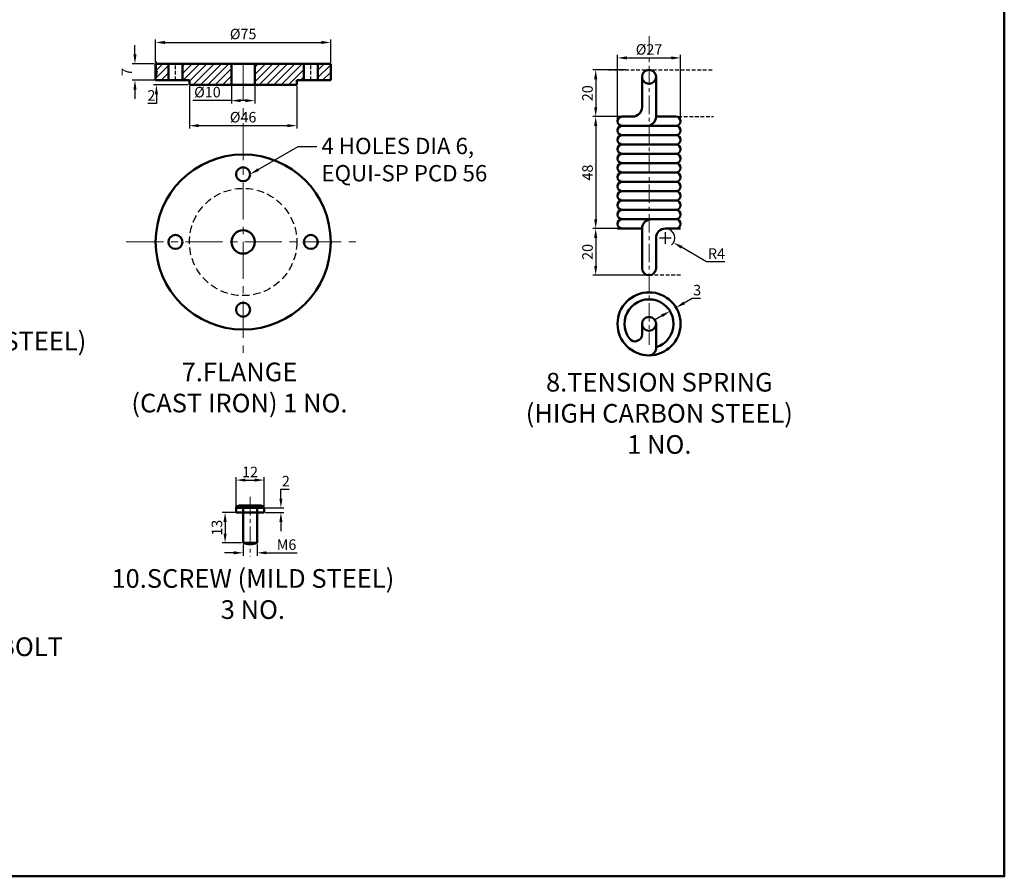
# Model space of a CAD drawing. Units: millimetres. Extents: x -166 to 681, y -4360 to 126.
# Tile 6 of 7: x 259 to 681, y -430 to -63. Entities that reach past the tile are written whole.
import ezdxf
from ezdxf import colors
from ezdxf.entities.mleader import LeaderData, LeaderLine
from ezdxf.math import Vec2, Vec3

# ---------------------------------------------------------------- set-up
doc = ezdxf.new("R2010")
doc.units = ezdxf.units.MM
doc.header["$LTSCALE"] = 0.5
doc.linetypes.add('CENTER', pattern=[50.8, 31.75, -6.35, 6.35, -6.35])
doc.linetypes.add('HIDDEN', pattern=[9.525, 6.35, -3.175])
for name, color, linetype, lineweight in [('M-CNTR', 1, 'CENTER', 18), ('M-DIMS', 2, 'Continuous', 25), ('M-HATC', 8, 'Continuous', 18), ('M-HIDN', 3, 'HIDDEN', 25), ('M-OUTL', 7, 'Continuous', 50), ('M-TEXT', 7, 'Continuous', 25), ('M-TTLB', 7, 'Continuous', 50)]:
    doc.layers.add(name, color=color, linetype=linetype, lineweight=lineweight)
doc.styles.get("Standard").update_dxf_attribs({"font": 'arial.ttf'})
doc.dimstyles.new('ISO-25', dxfattribs={"dimtxt": 4.5, "dimasz": 4, "dimexe": 1.25, "dimexo": 0.625, "dimtad": 1, "dimtoh": 1, "dimdec": 1, "dimtxsty": 'Standard', "dimcen": 2.5, "dimadec": 0, "dimazin": 0, "dimtfac": 1, "dimtdec": 1, "dimtofl": 0, "dimtmove": 0, "dimatfit": 3, "dimfxl": 1, "dimarcsym": 0})

# ---------------------------------------------------------------- blocks, each defined once
blk = doc.blocks.new('*D48')
at = {"layer": 'Defpoints', "color": 0, "ltscale": 0.5, "transparency": 16777216}
for p in [(392.3, -72.72), (317.3, -81.87), (392.3, -81.87)]:
    blk.add_point(p, dxfattribs=at)
at = {"layer": 'M-DIMS', "color": 0, "lineweight": -2, "ltscale": 0.5, "transparency": 16777216}
for p, q in [((317.3, -81.25), (317.3, -71.47)), ((392.3, -81.25), (392.3, -71.47)), ((321.3, -72.72), (388.3, -72.72))]:
    blk.add_line(p, q, dxfattribs=at)
at = {"layer": 'M-DIMS', "color": 0, "ltscale": 0.5, "transparency": 16777216}
for points in [[(321.3, -72.05), (321.3, -73.38), (317.3, -72.72)], [(388.3, -72.05), (388.3, -73.38), (392.3, -72.72)]]:
    blk.add_solid(points, dxfattribs=at)
at = {"layer": 'M-DIMS', "color": 0, "ltscale": 0.5, "transparency": 16777216, "insert": (354.8, -69.67), "char_height": 4.5, "attachment_point": 5}
blk.add_mtext('%%C75', dxfattribs=at)
blk = doc.blocks.new('*D49')
at = {"layer": 'Defpoints', "color": 0, "ltscale": 0.5, "transparency": 16777216}
for p in [(317.3, -81.87), (308.48, -88.87), (317.3, -88.87)]:
    blk.add_point(p, dxfattribs=at)
at = {"layer": 'M-DIMS', "color": 0, "lineweight": -2, "ltscale": 0.5, "transparency": 16777216}
for p, q in [((308.48, -77.87), (308.48, -73.87)), ((316.67, -81.87), (307.23, -81.87)), ((316.67, -88.87), (307.23, -88.87)), ((308.48, -92.87), (308.48, -96.87))]:
    blk.add_line(p, q, dxfattribs=at)
at = {"layer": 'M-DIMS', "color": 0, "ltscale": 0.5, "transparency": 16777216}
for points in [[(307.82, -77.87), (309.15, -77.87), (308.48, -81.87)], [(307.82, -92.87), (309.15, -92.87), (308.48, -88.87)]]:
    blk.add_solid(points, dxfattribs=at)
at = {"layer": 'M-DIMS', "color": 0, "ltscale": 0.5, "transparency": 16777216, "insert": (305.61, -85.37), "char_height": 4.5, "attachment_point": 5, "rotation": 90}
blk.add_mtext('7', dxfattribs=at)
blk = doc.blocks.new('*D50')
at = {"layer": 'Defpoints', "color": 0, "ltscale": 0.5, "transparency": 16777216}
for p in [(317.66, -90.87), (331.8, -88.87), (331.8, -90.87)]:
    blk.add_point(p, dxfattribs=at)
at = {"layer": 'M-DIMS', "color": 0, "lineweight": -2, "ltscale": 0.5, "transparency": 16777216}
for p, q in [((317.66, -84.87), (317.66, -80.87)), ((331.17, -88.87), (316.41, -88.87)), ((331.17, -90.87), (316.41, -90.87)), ((317.66, -94.87), (317.66, -98.87)), ((317.66, -98.87), (314.05, -98.87))]:
    blk.add_line(p, q, dxfattribs=at)
at = {"layer": 'M-DIMS', "color": 0, "ltscale": 0.5, "transparency": 16777216}
for points in [[(316.99, -84.87), (318.33, -84.87), (317.66, -88.87)], [(316.99, -94.87), (318.33, -94.87), (317.66, -90.87)]]:
    blk.add_solid(points, dxfattribs=at)
at = {"layer": 'M-DIMS', "color": 0, "ltscale": 0.5, "transparency": 16777216, "insert": (315.54, -95.99), "char_height": 4.5, "attachment_point": 5}
blk.add_mtext('2', dxfattribs=at)
blk = doc.blocks.new('*D51')
at = {"layer": 'Defpoints', "color": 0, "ltscale": 0.5, "transparency": 16777216}
for p in [(349.8, -90.87), (359.8, -90.87), (359.8, -97.63)]:
    blk.add_point(p, dxfattribs=at)
at = {"layer": 'M-DIMS', "color": 0, "lineweight": -2, "ltscale": 0.5, "transparency": 16777216}
for p, q in [((349.8, -91.5), (349.8, -98.88)), ((359.8, -91.5), (359.8, -98.88)), ((349.8, -97.63), (333.22, -97.63)), ((355.8, -97.63), (353.8, -97.63))]:
    blk.add_line(p, q, dxfattribs=at)
at = {"layer": 'M-DIMS', "color": 0, "ltscale": 0.5, "transparency": 16777216}
for points in [[(353.8, -96.97), (353.8, -98.3), (349.8, -97.63)], [(355.8, -96.97), (355.8, -98.3), (359.8, -97.63)]]:
    blk.add_solid(points, dxfattribs=at)
at = {"layer": 'M-DIMS', "color": 0, "ltscale": 0.5, "transparency": 16777216, "insert": (339.51, -94.58), "char_height": 4.5, "attachment_point": 5}
blk.add_mtext('%%C10', dxfattribs=at)
blk = doc.blocks.new('*D52')
at = {"layer": 'Defpoints', "color": 0, "ltscale": 0.5, "transparency": 16777216}
for p in [(331.8, -90.87), (377.8, -90.87), (377.8, -108.36)]:
    blk.add_point(p, dxfattribs=at)
at = {"layer": 'M-DIMS', "color": 0, "lineweight": -2, "ltscale": 0.5, "transparency": 16777216}
for p, q in [((331.8, -91.5), (331.8, -109.61)), ((377.8, -91.5), (377.8, -109.61)), ((335.8, -108.36), (373.8, -108.36))]:
    blk.add_line(p, q, dxfattribs=at)
at = {"layer": 'M-DIMS', "color": 0, "ltscale": 0.5, "transparency": 16777216}
for points in [[(335.8, -107.7), (335.8, -109.03), (331.8, -108.36)], [(373.8, -107.7), (373.8, -109.03), (377.8, -108.36)]]:
    blk.add_solid(points, dxfattribs=at)
at = {"layer": 'M-DIMS', "color": 0, "ltscale": 0.5, "transparency": 16777216, "insert": (354.8, -105.31), "char_height": 4.5, "attachment_point": 5}
blk.add_mtext('%%C46', dxfattribs=at)
blk = doc.blocks.new('*D55')
at = {"layer": 'Defpoints', "color": 0, "ltscale": 0.5, "transparency": 16777216}
for p in [(354.78, -274.15), (347.08, -287.15), (354.78, -287.15)]:
    blk.add_point(p, dxfattribs=at)
at = {"layer": 'M-DIMS', "color": 0, "lineweight": -2, "ltscale": 0.5, "transparency": 16777216}
for p, q in [((354.16, -274.15), (345.83, -274.15)), ((347.08, -278.15), (347.08, -283.15)), ((354.16, -287.15), (345.83, -287.15))]:
    blk.add_line(p, q, dxfattribs=at)
at = {"layer": 'M-DIMS', "color": 0, "ltscale": 0.5, "transparency": 16777216}
for points in [[(346.41, -278.15), (347.75, -278.15), (347.08, -274.15)], [(346.41, -283.15), (347.75, -283.15), (347.08, -287.15)]]:
    blk.add_solid(points, dxfattribs=at)
at = {"layer": 'M-DIMS', "color": 0, "ltscale": 0.5, "transparency": 16777216, "insert": (344.16, -280.65), "char_height": 4.5, "attachment_point": 5, "rotation": 90}
blk.add_mtext('13', dxfattribs=at)
blk = doc.blocks.new('*D56')
at = {"layer": 'Defpoints', "color": 0, "ltscale": 0.5, "transparency": 16777216}
for p in [(354.78, -287.15), (360.78, -287.15), (360.78, -291.39)]:
    blk.add_point(p, dxfattribs=at)
at = {"layer": 'M-DIMS', "color": 0, "lineweight": -2, "ltscale": 0.5, "transparency": 16777216}
for p, q in [((354.78, -287.77), (354.78, -292.64)), ((360.78, -287.77), (360.78, -292.64)), ((350.78, -291.39), (346.78, -291.39)), ((364.78, -291.39), (378.01, -291.39))]:
    blk.add_line(p, q, dxfattribs=at)
at = {"layer": 'M-DIMS', "color": 0, "ltscale": 0.5, "transparency": 16777216}
for points in [[(350.78, -290.72), (350.78, -292.06), (354.78, -291.39)], [(364.78, -290.72), (364.78, -292.06), (360.78, -291.39)]]:
    blk.add_solid(points, dxfattribs=at)
at = {"layer": 'M-DIMS', "color": 0, "ltscale": 0.5, "transparency": 16777216, "insert": (373.4, -288.47), "char_height": 4.5, "attachment_point": 5}
blk.add_mtext('M6', dxfattribs=at)
blk = doc.blocks.new('*D63')
at = {"layer": 'Defpoints', "color": 0, "ltscale": 0.5, "transparency": 16777216}
for p in [(542.14, -79.33), (515.14, -106.43), (542.14, -106.43)]:
    blk.add_point(p, dxfattribs=at)
at = {"layer": 'M-DIMS', "color": 0, "lineweight": -2, "ltscale": 0.5, "transparency": 16777216}
for p, q in [((515.14, -105.8), (515.14, -78.08)), ((519.14, -79.33), (538.14, -79.33)), ((542.14, -105.8), (542.14, -78.08))]:
    blk.add_line(p, q, dxfattribs=at)
at = {"layer": 'M-DIMS', "color": 0, "ltscale": 0.5, "transparency": 16777216}
for points in [[(519.14, -78.67), (519.14, -80), (515.14, -79.33)], [(538.14, -78.67), (538.14, -80), (542.14, -79.33)]]:
    blk.add_solid(points, dxfattribs=at)
at = {"layer": 'M-DIMS', "color": 0, "ltscale": 0.5, "transparency": 16777216, "insert": (528.64, -76.28), "char_height": 4.5, "attachment_point": 5}
blk.add_mtext('%%C27', dxfattribs=at)
blk = doc.blocks.new('*D64')
at = {"layer": 'Defpoints', "color": 0, "ltscale": 0.5, "transparency": 16777216}
for p in [(519.16, -84.46), (505.8, -104.46), (519.39, -104.46)]:
    blk.add_point(p, dxfattribs=at)
at = {"layer": 'M-DIMS', "color": 0, "lineweight": -2, "ltscale": 0.5, "transparency": 16777216}
for p, q in [((518.53, -84.46), (504.55, -84.46)), ((505.8, -88.46), (505.8, -100.46)), ((518.77, -104.46), (504.55, -104.46))]:
    blk.add_line(p, q, dxfattribs=at)
at = {"layer": 'M-DIMS', "color": 0, "ltscale": 0.5, "transparency": 16777216}
for points in [[(505.13, -88.46), (506.46, -88.46), (505.8, -84.46)], [(505.13, -100.46), (506.46, -100.46), (505.8, -104.46)]]:
    blk.add_solid(points, dxfattribs=at)
at = {"layer": 'M-DIMS', "color": 0, "ltscale": 0.5, "transparency": 16777216, "insert": (502.87, -94.46), "char_height": 4.5, "attachment_point": 5, "rotation": 90}
blk.add_mtext('20', dxfattribs=at)
blk = doc.blocks.new('*D65')
at = {"layer": 'Defpoints', "color": 0, "ltscale": 0.5, "transparency": 16777216}
for p in [(511.66, -104.46), (505.8, -152.46), (517.14, -152.46)]:
    blk.add_point(p, dxfattribs=at)
at = {"layer": 'M-DIMS', "color": 0, "lineweight": -2, "ltscale": 0.5, "transparency": 16777216}
for p, q in [((511.03, -104.46), (504.55, -104.46)), ((505.8, -108.46), (505.8, -148.46)), ((516.52, -152.46), (504.55, -152.46))]:
    blk.add_line(p, q, dxfattribs=at)
at = {"layer": 'M-DIMS', "color": 0, "ltscale": 0.5, "transparency": 16777216}
for points in [[(505.13, -108.46), (506.46, -108.46), (505.8, -104.46)], [(505.13, -148.46), (506.46, -148.46), (505.8, -152.46)]]:
    blk.add_solid(points, dxfattribs=at)
at = {"layer": 'M-DIMS', "color": 0, "ltscale": 0.5, "transparency": 16777216, "insert": (502.87, -128.46), "char_height": 4.5, "attachment_point": 5, "rotation": 90}
blk.add_mtext('48', dxfattribs=at)
blk = doc.blocks.new('*D66')
at = {"layer": 'Defpoints', "color": 0, "ltscale": 0.5, "transparency": 16777216}
for p in [(520.39, -152.46), (505.8, -172.46), (528.64, -172.46)]:
    blk.add_point(p, dxfattribs=at)
at = {"layer": 'M-DIMS', "color": 0, "lineweight": -2, "ltscale": 0.5, "transparency": 16777216}
for p, q in [((519.77, -152.46), (504.55, -152.46)), ((505.8, -156.46), (505.8, -168.46)), ((528.02, -172.46), (504.55, -172.46))]:
    blk.add_line(p, q, dxfattribs=at)
at = {"layer": 'M-DIMS', "color": 0, "ltscale": 0.5, "transparency": 16777216}
for points in [[(505.13, -156.46), (506.46, -156.46), (505.8, -152.46)], [(505.13, -168.46), (506.46, -168.46), (505.8, -172.46)]]:
    blk.add_solid(points, dxfattribs=at)
at = {"layer": 'M-DIMS', "color": 0, "ltscale": 0.5, "transparency": 16777216, "insert": (502.87, -162.46), "char_height": 4.5, "attachment_point": 5, "rotation": 90}
blk.add_mtext('20', dxfattribs=at)
blk = doc.blocks.new('*D67')
at = {"layer": 'Defpoints', "color": 0, "ltscale": 0.5, "transparency": 16777216}
for p in [(535.64, -156.46), (539.1, -158.46)]:
    blk.add_point(p, dxfattribs=at)
at = {"layer": 'M-DIMS', "color": 0, "lineweight": -2, "ltscale": 0.5, "transparency": 16777216}
for p, q in [((535.64, -158.96), (535.64, -153.96)), ((533.14, -156.46), (538.14, -156.46)), ((553.28, -166.64), (542.57, -160.46)), ((561.14, -166.64), (553.28, -166.64))]:
    blk.add_line(p, q, dxfattribs=at)
blk.add_arc((535.64, -156.46), 4, 312.0951, 81.0475, dxfattribs=at)
at = {"layer": 'M-DIMS', "color": 0, "ltscale": 0.5, "transparency": 16777216}
blk.add_solid([(542.9, -159.88), (542.24, -161.04), (539.1, -158.46)], dxfattribs=at)
at = {"layer": 'M-DIMS', "color": 0, "ltscale": 0.5, "transparency": 16777216, "insert": (557.52, -163.77), "char_height": 4.5, "attachment_point": 5}
blk.add_mtext('R4', dxfattribs=at)
blk = doc.blocks.new('*D68')
at = {"layer": 'Defpoints', "color": 0, "ltscale": 0.5, "transparency": 16777216}
for p in [(537.62, -187.84), (540.22, -186.34), (540.22, -186.34)]:
    blk.add_point(p, dxfattribs=at)
at = {"layer": 'M-DIMS', "color": 0, "lineweight": -2, "ltscale": 0.5, "transparency": 16777216}
for p, q in [((543.68, -184.34), (547.14, -182.34)), ((547.14, -182.34), (550.72, -182.34)), ((537.93, -188.38), (538.24, -188.92)), ((540.53, -186.88), (540.84, -187.42)), ((534.15, -189.84), (530.69, -191.84))]:
    blk.add_line(p, q, dxfattribs=at)
at = {"layer": 'M-DIMS', "color": 0, "ltscale": 0.5, "transparency": 16777216}
for points in [[(543.35, -183.76), (544.01, -184.91), (540.22, -186.34)], [(533.82, -189.26), (534.49, -190.41), (537.62, -187.84)]]:
    blk.add_solid(points, dxfattribs=at)
at = {"layer": 'M-DIMS', "color": 0, "ltscale": 0.5, "transparency": 16777216, "insert": (549.24, -179.41), "char_height": 4.5, "attachment_point": 5}
blk.add_mtext('3', dxfattribs=at)
blk = doc.blocks.new('*D87')
at = {"layer": 'Defpoints', "color": 0, "ltscale": 0.5, "transparency": 16777216}
for p in [(363.78, -260.23), (351.78, -274.15), (363.78, -274.15)]:
    blk.add_point(p, dxfattribs=at)
at = {"layer": 'M-DIMS', "color": 0, "lineweight": -2, "ltscale": 0.5, "transparency": 16777216}
for p, q in [((351.78, -273.52), (351.78, -258.98)), ((355.78, -260.23), (359.78, -260.23)), ((363.78, -273.52), (363.78, -258.98))]:
    blk.add_line(p, q, dxfattribs=at)
at = {"layer": 'M-DIMS', "color": 0, "ltscale": 0.5, "transparency": 16777216}
for points in [[(355.78, -259.56), (355.78, -260.89), (351.78, -260.23)], [(359.78, -259.56), (359.78, -260.89), (363.78, -260.23)]]:
    blk.add_solid(points, dxfattribs=at)
at = {"layer": 'M-DIMS', "color": 0, "ltscale": 0.5, "transparency": 16777216, "insert": (357.78, -257.34), "char_height": 4.5, "attachment_point": 5}
blk.add_mtext('12', dxfattribs=at)
blk = doc.blocks.new('*D88')
at = {"layer": 'Defpoints', "color": 0, "ltscale": 0.5, "transparency": 16777216}
for p in [(363.78, -272.15), (370.98, -272.15), (363.78, -274.15)]:
    blk.add_point(p, dxfattribs=at)
at = {"layer": 'M-DIMS', "color": 0, "lineweight": -2, "ltscale": 0.5, "transparency": 16777216}
for p, q in [((370.98, -268.15), (370.98, -264.15)), ((370.98, -264.15), (374.59, -264.15)), ((364.41, -272.15), (372.23, -272.15)), ((364.41, -274.15), (372.23, -274.15)), ((370.98, -278.15), (370.98, -282.15))]:
    blk.add_line(p, q, dxfattribs=at)
at = {"layer": 'M-DIMS', "color": 0, "ltscale": 0.5, "transparency": 16777216}
for points in [[(370.32, -268.15), (371.65, -268.15), (370.98, -272.15)], [(370.32, -278.15), (371.65, -278.15), (370.98, -274.15)]]:
    blk.add_solid(points, dxfattribs=at)
at = {"layer": 'M-DIMS', "color": 0, "ltscale": 0.5, "transparency": 16777216, "insert": (373.1, -261.26), "char_height": 4.5, "attachment_point": 5}
blk.add_mtext('2', dxfattribs=at)

msp = doc.modelspace()

# ---------------------------------------------------------------- hatches: boundary and pattern name
at = {"layer": 'M-HATC', "ltscale": 0.5}
h = msp.add_hatch(dxfattribs=at)
h.set_pattern_fill('ANSI31', color=256, scale=0.7)
h.set_pattern_definition([(45, (-558522.521, -290240.8901), (-1.571544821, 1.571544821), [])])
h.paths.add_polyline_path([(322.7995, -88.8706), (322.7995, -81.8706), (317.2995, -81.8706), (317.2995, -88.8706)])
h.paths.add_polyline_path([(349.7995, -90.8706), (349.7995, -81.8706), (328.7995, -81.8706), (328.7995, -88.8706), (331.7995, -88.8706), (331.7995, -90.8706)])
h.paths.add_polyline_path([(377.7995, -90.8706), (377.7995, -88.8706), (380.7995, -88.8706), (380.7995, -81.8706), (359.7995, -81.8706), (359.7995, -90.8706)])
h.paths.add_polyline_path([(392.2995, -81.8706), (386.7995, -81.8706), (386.7995, -88.8706), (392.2995, -88.8706)])

# ---------------------------------------------------------------- linework, layer by layer
at = {"layer": 'M-CNTR', "ltscale": 0.5}
for p, q in [((528.6407, -70.0538), (528.6407, -202.215)), ((357.782, -267.4267), (357.782, -292.9023))]:
    msp.add_line(p, q, dxfattribs=at)
at = {"layer": 'M-CNTR'}
for p, q in [((354.7995, -81.8706), (354.7995, -207.9941)), ((304.7638, -158.2074), (403.0861, -158.2074))]:
    msp.add_line(p, q, dxfattribs=at)
at = {"layer": 'M-HIDN', "ltscale": 0.5}
for p, q in [((325.7995, -88.8706), (325.7995, -81.8706)), ((383.7995, -88.8706), (383.7995, -81.8706)), ((511.2493, -84.46), (556.3137, -84.46)), ((531.6407, -104.46), (556.3137, -104.46)), ((542.1407, -172.46), (515.1407, -172.46))]:
    msp.add_line(p, q, dxfattribs=at)
at = {"layer": 'M-HIDN'}
msp.add_circle((354.7995, -158.2074), 23, dxfattribs=at)
at = {"layer": 'M-OUTL', "ltscale": 0.5}
for p, q in [((354.7995, -81.8706), (317.2995, -81.8706)), ((317.2995, -81.8706), (317.2995, -88.8706)), ((322.7995, -88.8706), (322.7995, -81.8706)), ((328.7995, -88.8706), (328.7995, -81.8706)), ((349.7995, -81.8706), (349.7995, -90.8706)), ((392.2995, -81.8706), (354.7995, -81.8706)), ((359.7995, -81.8706), (359.7995, -90.8706)), ((380.7995, -88.8706), (380.7995, -81.8706)), ((386.7995, -88.8706), (386.7995, -81.8706)), ((392.2995, -88.8706), (392.2995, -81.8706)), ((317.2995, -88.8706), (331.7995, -88.8706)), ((331.7995, -90.8706), (331.7995, -88.8706)), ((331.7995, -90.8706), (377.7995, -90.8706)), ((377.7995, -88.8706), (392.2995, -88.8706)), ((377.7995, -90.8706), (377.7995, -88.8706)), ((517.1407, -112.46), (540.1407, -112.46)), ((517.1407, -112.46), (540.1407, -112.46)), ((540.1407, -116.46), (517.1407, -116.46)), ((529.6407, -148.46), (540.1407, -148.46)), ((525.6407, -152.46), (515.1407, -152.46)), ((525.6407, -169.46), (525.6407, -152.46)), ((542.1407, -152.46), (535.6407, -152.46)), ((540.1407, -152.46), (535.6407, -152.46)), ((531.6407, -156.46), (531.6407, -169.46)), ((525.6407, -193.2829), (525.6407, -197.7829)), ((531.6407, -193.2829), (531.6407, -203.7829)), ((351.782, -274.1471), (351.782, -272.1471)), ((351.782, -272.1471), (363.782, -272.1471)), ((353.0418, -271.1471), (362.4992, -271.1471)), ((354.782, -287.1471), (354.782, -271.1471)), ((360.782, -287.1471), (360.782, -271.1471)), ((363.782, -272.1471), (363.782, -274.1471)), ((363.782, -274.1471), (351.782, -274.1471)), ((357.782, -287.1471), (354.782, -287.1471)), ((357.782, -287.1471), (360.782, -287.1471))]:
    msp.add_line(p, q, dxfattribs=at)
for points in [[(531.6407, -104.46), (540.1407, -104.46, -1), (540.1407, -108.46), (517.1407, -108.46, -1), (517.1407, -104.46), (521.6407, -104.46, 0.41421356), (525.6407, -100.46), (525.6407, -87.46)], [(517.1407, -108.46), (527.6407, -108.46, 0.41421356), (531.6407, -104.46), (531.6407, -87.46)]]:
    msp.add_lwpolyline(points, format="xyb", dxfattribs=at)
for points in [[(517.1407, -116.46), (540.1407, -116.46, -1), (540.1407, -120.46), (517.1407, -120.46, -1)], [(517.1407, -120.46), (540.1407, -120.46, -1), (540.1407, -124.46), (517.1407, -124.46, -1)], [(517.1407, -124.46), (540.1407, -124.46, -1), (540.1407, -128.46), (517.1407, -128.46, -1)], [(517.1407, -128.46), (540.1407, -128.46, -1), (540.1407, -132.46), (517.1407, -132.46, -1)], [(517.1407, -132.46), (540.1407, -132.46, -1), (540.1407, -136.46), (517.1407, -136.46, -1)], [(517.1407, -136.46), (540.1407, -136.46, -1), (540.1407, -140.46), (517.1407, -140.46, -1)], [(517.1407, -140.46), (540.1407, -140.46, -1), (540.1407, -144.46), (517.1407, -144.46, -1)], [(517.1407, -144.46), (540.1407, -144.46, -1), (540.1407, -148.46), (517.1407, -148.46, -1)]]:
    msp.add_lwpolyline(points, format="xyb", close=True, dxfattribs=at)
for centre, radius in [((528.6407, -87.46), 3), ((528.6407, -193.2829), 13.5), ((528.6407, -193.2829), 3)]:
    msp.add_circle(centre, radius, dxfattribs=at)
at = {"layer": 'M-OUTL'}
for centre, radius in [((354.7995, -158.2074), 37.5), ((354.7995, -129.2074), 3), ((325.7995, -158.2074), 3), ((354.7995, -158.2074), 5), ((383.7995, -158.2074), 3), ((354.7995, -187.2074), 3)]:
    msp.add_circle(centre, radius, dxfattribs=at)
at = {"layer": 'M-OUTL', "ltscale": 0.5}
for centre, radius, start, end in [((517.1407, -110.46), 2, 90, 270), ((540.1407, -110.46), 2, 270, 90), ((517.1407, -114.46), 2, 90, 270), ((540.1407, -114.46), 2, 270, 90), ((517.1407, -150.46), 2, 90, 270), ((529.6407, -152.46), 4, 90, 180), ((540.1407, -150.46), 2, 270, 90), ((535.6407, -156.46), 4, 90, 180), ((528.6407, -169.46), 3, 180, 0), ((528.6407, -193.2829), 10.5, 286.60155, 216.869898), ((522.6407, -197.7829), 3, 216.869898, 0), ((528.6407, -203.7829), 3, 270, 0), ((353.282, -272.7432), 1.6141, 21.6745, 158.3255), ((357.782, -276.1471), 5, 53.130102, 126.869898), ((362.282, -272.7485), 1.6161, 21.847759, 158.152241), ((357.782, -279.9866), 7.7635, 247.267941, 292.732059)]:
    msp.add_arc(centre, radius, start, end, dxfattribs=at)
at = {"layer": 'M-TTLB', "ltscale": 0.5}
msp.add_lwpolyline([(-165.9437, 126.0872), (680.7907, 126.0872), (680.7907, -430.0081), (-165.9437, -430.0081)], close=True, dxfattribs=at)

# ---------------------------------------------------------------- texts
at = {"layer": 'M-TEXT', "ltscale": 0.5, "char_height": 8, "attachment_point": 1}
for s, insert in [('\\pxqc;6.STEM (MILD STEEL) \\P1 NO.', (158.6774, -196.6773)), ('\\pxqc;7.FLANGE\\P(CAST IRON) 1 NO.', (277.7691, -209.8893)), ('\\pxqc;8.TENSION SPRING\\P(HIGH CARBON STEEL) \\P1 NO.', (457.573, -214.2937)), ('\\pxqc;10.SCREW (MILD STEEL) \\P3 NO.', (283.5156, -298.3817)), ('\\pxqc;9.TENSION ADJUSTING BOLT WITH NUT\\P(MILD STEEL) \\P1 NO.', (128.2808, -327.6326))]:
    msp.add_mtext_dynamic_manual_height_columns(s, width=150.92987, gutter_width=12.5, heights=[0], dxfattribs=dict(at, insert=insert))

# ---------------------------------------------------------------- dimensions: what is measured, and where the dimension line sits
at = {"layer": 'M-DIMS', "ltscale": 0.5}
for base, p1, p2, picture, middle in [((392.2995, -72.7181), (317.2995, -81.8706), (392.2995, -81.8706), '*D48', (354.7995, -69.6697)), ((542.1405, -79.3325), (515.141, -106.4279), (542.1405, -106.4279), '*D63', (528.6407, -76.284)), ((377.7995, -108.3625), (331.7995, -90.8706), (377.7995, -90.8706), '*D52', (354.7995, -105.3141))]:
    dim = msp.add_linear_dim(base=base, p1=p1, p2=p2, text='%%C<>', dimstyle='ISO-25', override={"dimclrd": 0, "dimclre": 0, "dimclrt": 0}, dxfattribs=at)
    dim.commit()
    dim.dimension.update_dxf_attribs({"geometry": picture, "text_midpoint": middle})
for base, p1, p2, override, picture, middle in [((308.4831, -88.8706), (317.2995, -81.8706), (317.2995, -88.8706), {"dimclrd": 0, "dimclre": 0, "dimclrt": 0}, '*D49', (305.6081, -85.3706)), ((317.6601, -90.8706), (331.7995, -88.8706), (331.7995, -90.8706), {"dimclrd": 0, "dimclre": 0, "dimclrt": 0}, '*D50', (315.5449, -95.9864)), ((505.7951, -104.46), (519.1584, -84.46), (519.3907, -104.46), {"dimclrd": 0, "dimclre": 0, "dimclrt": 0}, '*D64', (502.8725, -94.46)), ((505.7951, -152.46), (511.6554, -104.46), (517.1407, -152.46), {"dimclrd": 0, "dimclre": 0, "dimclrt": 0}, '*D65', (502.8725, -128.46)), ((505.7951, -172.46), (520.3907, -152.46), (528.6407, -172.46), {"dimclrd": 0, "dimclre": 0, "dimclrt": 0}, '*D66', (502.8725, -162.46)), ((370.982, -272.1471), (363.782, -274.1471), (363.782, -272.1471), {"dimdec": 0, "dimlfac": 1, "dimrnd": 0, "dimzin": 0, "dimdsep": 46, "dimlunit": 2}, '*D88', (373.0973, -261.2629)), ((347.0811, -287.1471), (354.782, -274.1471), (354.782, -287.1471), {"dimclrd": 0, "dimclre": 0, "dimclrt": 0}, '*D55', (344.157, -280.6471))]:
    dim = msp.add_linear_dim(base=base, p1=p1, p2=p2, angle=90, dimstyle='ISO-25', override=override, dxfattribs=at)
    dim.commit()
    dim.dimension.update_dxf_attribs({"geometry": picture, "text_midpoint": middle})
for base, p1, p2, text, picture, middle in [((359.7995, -97.6324), (349.7995, -90.8706), (359.7995, -90.8706), '%%C<>', '*D51', (339.5111, -97.6324)), ((360.782, -291.3891), (354.782, -287.1471), (360.782, -287.1471), 'M<>', '*D56', (373.3959, -291.3891))]:
    dim = msp.add_linear_dim(base=base, p1=p1, p2=p2, text=text, dimstyle='ISO-25', override={"dimclrd": 0, "dimclre": 0, "dimclrt": 0}, dxfattribs=at)
    dim.commit()
    dim.dimension.update_dxf_attribs({"geometry": picture, "text_midpoint": middle, "dimtype": 160})
dim = msp.add_radius_dim(center=(535.6407, -156.46), mpoint=(539.1048, -158.46), dimstyle='ISO-25', override={"dimclrd": 0, "dimclre": 0, "dimclrt": 0}, dxfattribs=at)
dim.commit()
dim.dimension.update_dxf_attribs({"geometry": '*D67', "text_midpoint": (557.5206, -166.642), "dimtype": 164})
dim = msp.add_aligned_dim(p1=(537.6177, -187.8365), p2=(540.2163, -186.3362), distance=0, dimstyle='ISO-25', override={"dimclrd": 0, "dimclre": 0, "dimclrt": 0}, dxfattribs=at)
dim.commit()
dim.dimension.update_dxf_attribs({"geometry": '*D68', "text_midpoint": (549.2429, -179.4121)})
dim = msp.add_linear_dim(base=(363.782, -260.2267), p1=(351.782, -274.1471), p2=(363.782, -274.1471), dimstyle='ISO-25', override={"dimdec": 0, "dimlfac": 1, "dimrnd": 0, "dimzin": 0, "dimdsep": 46, "dimlunit": 2}, dxfattribs=at)
dim.commit()
dim.dimension.update_dxf_attribs({"geometry": '*D87', "text_midpoint": (357.782, -257.3425)})

# ---------------------------------------------------------------- leaders
at = {"layer": 'M-TEXT', "ltscale": 0.5}
ml = msp.add_multileader_mtext('Standard', dxfattribs=at)
ml.set_content('4 HOLES DIA 6,\\PEQUI-SP PCD 56', color=256)
ml.set_leader_properties()
ml.build(insert=Vec2(0, 0))
ctx = ml.context
ctx.base_point, ctx.char_height, ctx.plane_origin = Vec3(386.3411, -117.3476), 7, Vec3(357.7995, -129.2074)
notes = []
notes.append((ctx, [(0, (1, 1, 0), (378.3411, -117.3476), (1, 0), 8, [(0, [(357.7995, -129.2074)], 0, [])])]))
ctx.mtext.insert, ctx.mtext.flow_direction = Vec3(388.3411, -113.5754), 5
for ctx, leaders in notes:
    for number, flags, end, landing, length, lines in leaders:
        leader = LeaderData()
        leader.index, (leader.has_last_leader_line, leader.has_dogleg_vector, leader.attachment_direction) = number, flags
        leader.last_leader_point, leader.dogleg_vector, leader.dogleg_length = Vec3(end), Vec3(landing), length
        for number, points, colour, breaks in lines:
            line = LeaderLine()
            line.index, line.vertices, line.color, line.breaks = number, Vec3.list(points), colors.encode_raw_color(colour), breaks
            leader.lines.append(line)
        ctx.leaders.append(leader)

doc.saveas('drawing.dxf')
